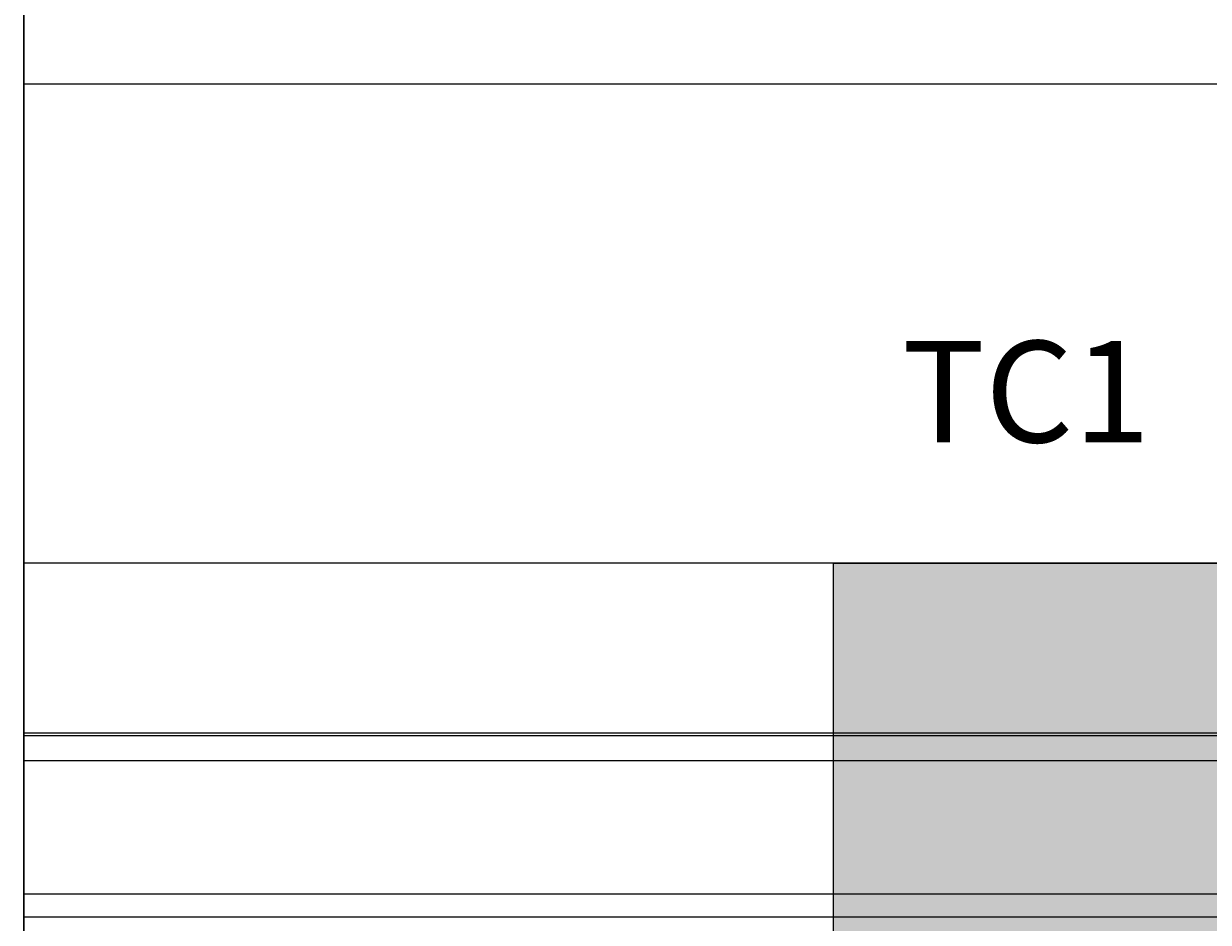
# Model space of a CAD drawing. Units: inches. Extents: x 35362 to 73946, y 43607 to 67532.
# Tile 4 of 134: x 35362 to 37937, y 48909 to 50863. Entities that reach past the tile are written whole.
import ezdxf

# ---------------------------------------------------------------- set-up
doc = ezdxf.new("R2010")
doc.units = ezdxf.units.IN
doc.header["$MEASUREMENT"] = 0
for name, color, linetype, lineweight in [('A-ANNO-DIMS', 2, 'Continuous', 18), ('E-ANNO-TEXT', 5, 'Continuous', 18), ('E-SYMB', 1, 'Continuous', 25), ('E-SYMB-PATT', 1, 'Continuous', 13)]:
    doc.layers.add(name, color=color, linetype=linetype, lineweight=lineweight)
doc.styles.get("Standard").update_dxf_attribs({"font": 'arial.ttf'})
doc.dimstyles.get("Standard").update_dxf_attribs({"dimtxt": 0.18, "dimasz": 0.18, "dimexe": 0.18, "dimexo": 0.0625, "dimgap": 0.09, "dimtad": 0, "dimtih": 1, "dimtoh": 1, "dimdec": 4, "dimzin": 0, "dimdsep": 46, "dimtxsty": 'Standard', "dimcen": 0.09, "dimadec": 0, "dimazin": 0, "dimtfac": 1, "dimtdec": 4, "dimtofl": 0, "dimtmove": 0, "dimatfit": 3, "dimfxl": 1, "dimtolj": 1, "dimtzin": 0, "dimarcsym": 0})

# ---------------------------------------------------------------- blocks, each defined once
blk = doc.blocks.new('*D16')
at = {"layer": 'A-ANNO-DIMS', "color": 0, "lineweight": -2, "transparency": 16777216}
for p, q in [((37121.9, 49689.8), (35361.8, 49689.8)), ((35361.9, 49689.7), (35361.9, 48304.8)), ((35361.9, 46919.6), (35361.9, 48304.4)), ((37121.9, 46919.4), (35361.8, 46919.4))]:
    blk.add_line(p, q, dxfattribs=at)
at = {"layer": 'A-ANNO-DIMS', "color": 0, "transparency": 16777216}
for points in [[(35361.9, 49689.7), (35362, 49689.7), (35361.9, 49689.8)], [(35361.9, 46919.6), (35362, 46919.6), (35361.9, 46919.4)]]:
    blk.add_solid(points, dxfattribs=at)
at = {"layer": 'Defpoints', "color": 0, "transparency": 16777216}
for p in [(37121.9, 49689.8), (35361.9, 46919.4), (37121.9, 46919.4)]:
    blk.add_point(p, dxfattribs=at)
at = {"layer": 'A-ANNO-DIMS', "color": 0, "transparency": 16777216, "insert": (35361.9, 48304.6), "char_height": 0.18, "attachment_point": 5}
blk.add_mtext('\\A1;2770.5', dxfattribs=at)
blk = doc.blocks.new('*D40')
at = {"layer": 'A-ANNO-DIMS', "color": 0, "lineweight": -2, "transparency": 16777216}
for p, q in [((56873.5, 53351.5), (35361.8, 53351.5)), ((35361.9, 53351.3), (35361.9, 51333.3)), ((35361.9, 49314.8), (35361.9, 51332.9)), ((51806.5, 49314.7), (35361.8, 49314.7))]:
    blk.add_line(p, q, dxfattribs=at)
at = {"layer": 'A-ANNO-DIMS', "color": 0, "transparency": 16777216}
for points in [[(35361.9, 53351.3), (35362, 53351.3), (35361.9, 53351.5)], [(35361.9, 49314.8), (35362, 49314.8), (35361.9, 49314.7)]]:
    blk.add_solid(points, dxfattribs=at)
at = {"layer": 'Defpoints', "color": 0, "transparency": 16777216}
for p in [(35361.9, 53351.5), (56873.6, 53351.5), (51806.5, 49314.7)]:
    blk.add_point(p, dxfattribs=at)
at = {"layer": 'A-ANNO-DIMS', "color": 0, "transparency": 16777216, "insert": (35361.9, 51333.1), "char_height": 0.18, "attachment_point": 5}
blk.add_mtext('\\A1;4036.9', dxfattribs=at)
blk = doc.blocks.new('*D58')
at = {"layer": 'A-ANNO-DIMS', "color": 0, "lineweight": -2, "transparency": 16777216}
for p, q in [((38575.7, 50731.8), (35361.8, 50731.8)), ((35361.9, 50731.6), (35361.9, 50211)), ((35361.9, 49690), (35361.9, 50210.7)), ((38575.7, 49689.8), (35361.8, 49689.8))]:
    blk.add_line(p, q, dxfattribs=at)
at = {"layer": 'A-ANNO-DIMS', "color": 0, "transparency": 16777216}
for points in [[(35361.9, 50731.6), (35362, 50731.6), (35361.9, 50731.8)], [(35361.9, 49690), (35362, 49690), (35361.9, 49689.8)]]:
    blk.add_solid(points, dxfattribs=at)
at = {"layer": 'Defpoints', "color": 0, "transparency": 16777216}
for p in [(38575.8, 50731.8), (35361.9, 49689.8), (38575.8, 49689.8)]:
    blk.add_point(p, dxfattribs=at)
at = {"layer": 'A-ANNO-DIMS', "color": 0, "transparency": 16777216, "insert": (35361.9, 50210.8), "char_height": 0.18, "attachment_point": 5}
blk.add_mtext('\\A1;1042.0', dxfattribs=at)
blk = doc.blocks.new('*D67')
at = {"layer": 'A-ANNO-DIMS', "color": 0, "lineweight": -2, "transparency": 16777216}
for p, q in [((56873.5, 53351.5), (35361.8, 53351.5)), ((35361.9, 53351.3), (35361.9, 49400.9)), ((35361.9, 45450.1), (35361.9, 49400.5)), ((53793.6, 45449.9), (35361.8, 45449.9))]:
    blk.add_line(p, q, dxfattribs=at)
at = {"layer": 'A-ANNO-DIMS', "color": 0, "transparency": 16777216}
for points in [[(35361.9, 53351.3), (35362, 53351.3), (35361.9, 53351.5)], [(35361.9, 45450.1), (35362, 45450.1), (35361.9, 45449.9)]]:
    blk.add_solid(points, dxfattribs=at)
at = {"layer": 'Defpoints', "color": 0, "transparency": 16777216}
for p in [(35361.9, 53351.5), (56873.6, 53351.5), (53793.6, 45449.9)]:
    blk.add_point(p, dxfattribs=at)
at = {"layer": 'A-ANNO-DIMS', "color": 0, "transparency": 16777216, "insert": (35361.9, 49400.7), "char_height": 0.18, "attachment_point": 5}
blk.add_mtext('\\A1;7901.6', dxfattribs=at)
blk = doc.blocks.new('*D84')
at = {"layer": 'A-ANNO-DIMS', "color": 0, "lineweight": -2, "transparency": 16777216}
for p, q in [((55540.2, 49259.9), (35361.8, 49259.9)), ((35361.9, 49259.8), (35361.9, 49115.1)), ((35361.9, 48970.2), (35361.9, 49114.8)), ((55540.2, 48970), (35361.8, 48970))]:
    blk.add_line(p, q, dxfattribs=at)
at = {"layer": 'A-ANNO-DIMS', "color": 0, "transparency": 16777216}
for points in [[(35361.9, 49259.8), (35362, 49259.8), (35361.9, 49259.9)], [(35361.9, 48970.2), (35362, 48970.2), (35361.9, 48970)]]:
    blk.add_solid(points, dxfattribs=at)
at = {"layer": 'Defpoints', "color": 0, "transparency": 16777216}
for p in [(35361.9, 49259.9), (55540.3, 49259.9), (55540.3, 48970)]:
    blk.add_point(p, dxfattribs=at)
at = {"layer": 'A-ANNO-DIMS', "color": 0, "transparency": 16777216, "insert": (35361.9, 49115), "char_height": 0.18, "attachment_point": 5}
blk.add_mtext('\\A1;289.96', dxfattribs=at)
blk = doc.blocks.new('*D86')
at = {"layer": 'A-ANNO-DIMS', "color": 0, "lineweight": -2, "transparency": 16777216}
for p, q in [((51285.5, 49320.1), (35361.8, 49320.1)), ((35361.9, 49319.9), (35361.9, 49120.3)), ((35361.9, 48920.3), (35361.9, 49119.9)), ((51285.5, 48920.1), (35361.8, 48920.1))]:
    blk.add_line(p, q, dxfattribs=at)
at = {"layer": 'A-ANNO-DIMS', "color": 0, "transparency": 16777216}
for points in [[(35361.9, 49319.9), (35362, 49319.9), (35361.9, 49320.1)], [(35361.9, 48920.3), (35362, 48920.3), (35361.9, 48920.1)]]:
    blk.add_solid(points, dxfattribs=at)
at = {"layer": 'Defpoints', "color": 0, "transparency": 16777216}
for p in [(35361.9, 49320.1), (51285.6, 49320.1), (51285.6, 48920.1)]:
    blk.add_point(p, dxfattribs=at)
at = {"layer": 'A-ANNO-DIMS', "color": 0, "transparency": 16777216, "insert": (35361.9, 49120.1), "char_height": 0.18, "attachment_point": 5}
blk.add_mtext('\\A1;400.0', dxfattribs=at)

msp = doc.modelspace()

# ---------------------------------------------------------------- hatches: boundary and pattern name
at = {"layer": 'E-SYMB-PATT'}
h = msp.add_hatch(color=256, dxfattribs=at)
h.dxf.hatch_style = 1
h.paths.add_polyline_path([(39894.84, 49689.843), (37121.949, 49689.843), (37121.949, 46919.381), (39894.84, 46919.381)])

# ---------------------------------------------------------------- linework, layer by layer
at = {"layer": 'E-SYMB'}
msp.add_lwpolyline([(37121.949, 49689.843), (39894.84, 49689.843), (39894.84, 46919.381), (37121.949, 46919.381)], close=True, dxfattribs=at)

# ---------------------------------------------------------------- texts
at = {"layer": 'E-ANNO-TEXT'}
msp.add_text('TC1', height=220.866, dxfattribs=at).set_placement((37271.324, 49952.699))

# ---------------------------------------------------------------- dimensions: what is measured, and where the dimension line sits
at = {"layer": 'A-ANNO-DIMS'}
for base, p1, p2, override, picture, middle in [((35361.949, 53351.529), (51806.517, 49314.669), (56873.602, 53351.529), {"dimdec": 1, "dimlfac": 1, "dimrnd": 0, "dimzin": 0, "dimdsep": 46, "dimlunit": 2}, '*D40', (35361.949, 51333.099)), ((35361.949, 53351.529), (53793.638, 45449.894), (56873.602, 53351.529), {"dimdec": 1, "dimlfac": 1, "dimrnd": 0, "dimzin": 0, "dimdsep": 46, "dimlunit": 2}, '*D67', (35361.949, 49400.712)), ((35361.949, 49689.843), (38575.774, 50731.821), (38575.774, 49689.843), {"dimdec": 1, "dimlfac": 1, "dimrnd": 0, "dimzin": 0, "dimdsep": 46, "dimlunit": 2}, '*D58', (35361.949, 50210.832)), ((35361.949, 46919.381), (37121.949, 49689.843), (37121.949, 46919.381), {"dimdec": 1, "dimlfac": 1, "dimrnd": 0, "dimzin": 0, "dimdsep": 46, "dimlunit": 2}, '*D16', (35361.949, 48304.612)), ((35361.949, 49320.079), (51285.595, 48920.079), (51285.595, 49320.079), {"dimdec": 1, "dimlfac": 1, "dimrnd": 0, "dimzin": 0, "dimdsep": 46, "dimlunit": 2}, '*D86', (35361.949, 49120.079)), ((35361.9491, 49259.9353), (55540.2972, 48969.9796), (55540.2972, 49259.9353), {"dimdec": 2, "dimlfac": 1, "dimrnd": 0, "dimzin": 0, "dimdsep": 46, "dimlunit": 2}, '*D84', (35361.9491, 49114.9575))]:
    dim = msp.add_linear_dim(base=base, p1=p1, p2=p2, angle=90, dimstyle='Standard', override=override, dxfattribs=at)
    dim.commit()
    dim.dimension.update_dxf_attribs({"geometry": picture, "text_midpoint": middle})

doc.saveas('drawing.dxf')
